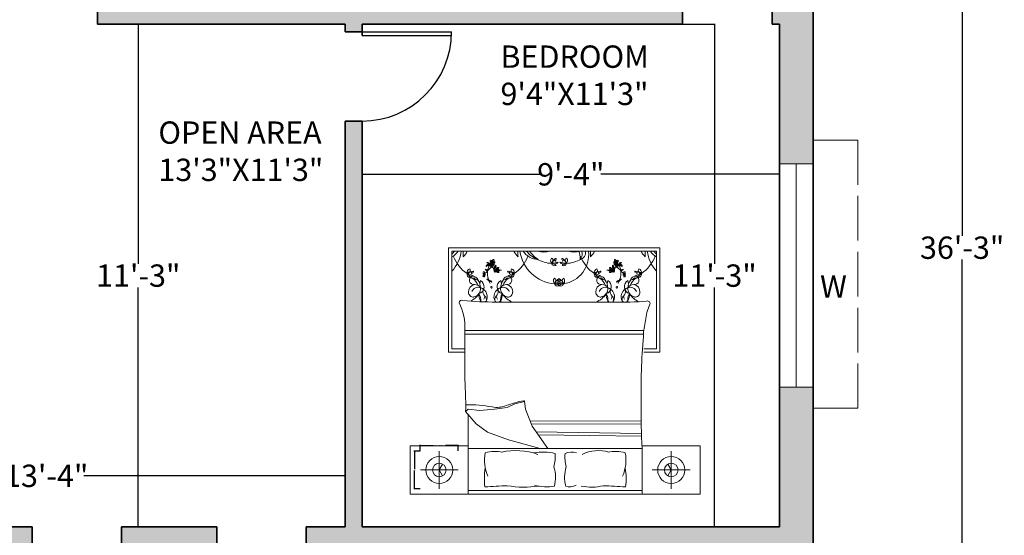
# Model space of a CAD drawing. Units: inches. Extents: x -5 to 482, y -460 to 66.
# Tile 16 of 31: x 218 to 482, y -282 to -143. Entities that reach past the tile are written whole.
import ezdxf

# ---------------------------------------------------------------- set-up
doc = ezdxf.new("R2010")
doc.units = ezdxf.units.IN
doc.header["$MEASUREMENT"] = 0
doc.linetypes.add('ACAD_ISO02W100', pattern=[15, 12, -3])
for name, color, linetype, lineweight in [('A-ANNO-DIMS', 2, 'Continuous', 18), ('A-ANNO-TEXT', 7, 'Continuous', 18), ('A-AREA-IDEN', 7, 'Continuous', 18), ('A-DOOR', 3, 'Continuous', 25), ('A-FURN', 8, 'Continuous', 18), ('A-GLAZ', 4, 'Continuous', 18), ('A-GLAZ-OVHD', 4, 'ACAD_ISO02W100', 13), ('A-WALL', 7, 'Continuous', 35), ('A-WALL-PATT', 152, 'Continuous', 13)]:
    doc.layers.add(name, color=color, linetype=linetype, lineweight=lineweight)
doc.styles.get("Standard").update_dxf_attribs({"font": 'arial.ttf'})
doc.dimstyles.get("Standard").update_dxf_attribs({"dimtxt": 0.18, "dimasz": 0.18, "dimexe": 0.18, "dimexo": 0.0625, "dimgap": 0.09, "dimtad": 0, "dimtih": 1, "dimtoh": 1, "dimdec": 0, "dimzin": 0, "dimdsep": 46, "dimlunit": 3, "dimtxsty": 'Standard', "dimcen": 0.09, "dimadec": 0, "dimazin": 0, "dimtfac": 1, "dimtdec": 0, "dimtofl": 0, "dimtmove": 0, "dimatfit": 3, "dimfxl": 1, "dimtolj": 1, "dimtzin": 0, "dimarcsym": 0})

# ---------------------------------------------------------------- blocks, each defined once
blk = doc.blocks.new('*D4')
at = {"layer": 'A-ANNO-DIMS', "color": 0, "lineweight": -2, "transparency": 16777216}
for p, q in [((430.44, 13.15), (470.55, 13.15)), ((470.37, 12.97), (470.37, -201.19)), ((470.37, -421.67), (470.37, -207.5)), ((430.44, -421.85), (470.55, -421.85))]:
    blk.add_line(p, q, dxfattribs=at)
at = {"layer": 'A-ANNO-DIMS', "color": 0, "transparency": 16777216}
for points in [[(470.34, 12.97), (470.4, 12.97), (470.37, 13.15)], [(470.34, -421.67), (470.4, -421.67), (470.37, -421.85)]]:
    blk.add_solid(points, dxfattribs=at)
at = {"layer": 'Defpoints', "color": 0, "transparency": 16777216}
for p in [(430.38, 13.15), (430.38, -421.85), (470.37, -421.85)]:
    blk.add_point(p, dxfattribs=at)
at = {"layer": 'A-ANNO-DIMS', "color": 0, "transparency": 16777216, "insert": (470.37, -204.35), "char_height": 6, "attachment_point": 5}
blk.add_mtext('\\A1;36\'-3"', dxfattribs=at)
blk = doc.blocks.new('*D15')
at = {"layer": 'A-ANNO-DIMS', "color": 0, "lineweight": -2, "transparency": 16777216}
for p, q in [((309.38, -184.91), (309.38, -184.46)), ((309.56, -184.64), (357.31, -184.64)), ((421.2, -184.64), (373.44, -184.64)), ((421.38, -184.91), (421.38, -184.46))]:
    blk.add_line(p, q, dxfattribs=at)
at = {"layer": 'A-ANNO-DIMS', "color": 0, "transparency": 16777216}
for points in [[(309.56, -184.61), (309.56, -184.67), (309.38, -184.64)], [(421.2, -184.61), (421.2, -184.67), (421.38, -184.64)]]:
    blk.add_solid(points, dxfattribs=at)
at = {"layer": 'Defpoints', "color": 0, "transparency": 16777216}
for p in [(421.38, -184.64), (309.38, -184.98), (421.38, -184.98)]:
    blk.add_point(p, dxfattribs=at)
at = {"layer": 'A-ANNO-DIMS', "color": 0, "transparency": 16777216, "insert": (365.38, -184.64), "char_height": 6, "attachment_point": 5}
blk.add_mtext('\\A1;9\'-4"', dxfattribs=at)
blk = doc.blocks.new('*D16')
at = {"layer": 'A-ANNO-DIMS', "color": 0, "lineweight": -2, "transparency": 16777216}
for p, q in [((395.44, -144.35), (404.13, -144.35)), ((403.95, -144.53), (403.95, -208.69)), ((403.95, -279.17), (403.95, -215)), ((395.44, -279.35), (404.13, -279.35))]:
    blk.add_line(p, q, dxfattribs=at)
at = {"layer": 'A-ANNO-DIMS', "color": 0, "transparency": 16777216}
for points in [[(403.92, -144.53), (403.98, -144.53), (403.95, -144.35)], [(403.92, -279.17), (403.98, -279.17), (403.95, -279.35)]]:
    blk.add_solid(points, dxfattribs=at)
at = {"layer": 'Defpoints', "color": 0, "transparency": 16777216}
for p in [(395.38, -144.35), (395.38, -279.35), (403.95, -279.35)]:
    blk.add_point(p, dxfattribs=at)
at = {"layer": 'A-ANNO-DIMS', "color": 0, "transparency": 16777216, "insert": (403.95, -211.85), "char_height": 6, "attachment_point": 5}
blk.add_mtext('\\A1;11\'-3"', dxfattribs=at)
blk = doc.blocks.new('*D17')
at = {"layer": 'A-ANNO-DIMS', "color": 0, "lineweight": -2, "transparency": 16777216}
for p, q in [((238.44, -144.35), (249.52, -144.35)), ((249.34, -144.53), (249.34, -208.69)), ((249.34, -279.17), (249.34, -215)), ((244.94, -279.35), (249.52, -279.35))]:
    blk.add_line(p, q, dxfattribs=at)
at = {"layer": 'A-ANNO-DIMS', "color": 0, "transparency": 16777216}
for points in [[(249.31, -144.53), (249.37, -144.53), (249.34, -144.35)], [(249.31, -279.17), (249.37, -279.17), (249.34, -279.35)]]:
    blk.add_solid(points, dxfattribs=at)
at = {"layer": 'Defpoints', "color": 0, "transparency": 16777216}
for p in [(238.38, -144.35), (244.88, -279.35), (249.34, -279.35)]:
    blk.add_point(p, dxfattribs=at)
at = {"layer": 'A-ANNO-DIMS', "color": 0, "transparency": 16777216, "insert": (249.34, -211.85), "char_height": 6, "attachment_point": 5}
blk.add_mtext('\\A1;11\'-3"', dxfattribs=at)
blk = doc.blocks.new('*D20')
at = {"layer": 'A-ANNO-DIMS', "color": 0, "lineweight": -2, "transparency": 16777216}
for p, q in [((144.41, -279.11), (144.41, -265.44)), ((144.59, -265.62), (214.53, -265.62)), ((304.7, -265.62), (234.75, -265.62)), ((304.88, -279.11), (304.88, -265.44))]:
    blk.add_line(p, q, dxfattribs=at)
at = {"layer": 'A-ANNO-DIMS', "color": 0, "transparency": 16777216}
for points in [[(144.59, -265.59), (144.59, -265.65), (144.41, -265.62)], [(304.7, -265.59), (304.7, -265.65), (304.88, -265.62)]]:
    blk.add_solid(points, dxfattribs=at)
at = {"layer": 'Defpoints', "color": 0, "transparency": 16777216}
for p in [(304.88, -265.62), (144.41, -279.17), (304.88, -279.17)]:
    blk.add_point(p, dxfattribs=at)
at = {"layer": 'A-ANNO-DIMS', "color": 0, "transparency": 16777216, "insert": (224.64, -265.62), "char_height": 6, "attachment_point": 5}
blk.add_mtext('\\A1;13\'-4"', dxfattribs=at)
blk = doc.blocks.new('DOOR-SWING-24IN')
for p, q in [((24, 1), (0, 1)), ((24, 0), (0, 0))]:
    blk.add_line(p, q)
blk.add_arc((24, 0), 24, 90, 180)
blk = doc.blocks.new('WIN-GLAZ-60IN')
for p, q in [((0, 9), (60, 9)), ((0, 4.5), (60, 4.5)), ((60, 0), (0, 0))]:
    blk.add_line(p, q)
blk = doc.blocks.new('WIN-SHADE-72IN')
for p, q in [((0, 12), (72, 12)), ((0, 12), (0, 0)), ((72, 12), (72, 0))]:
    blk.add_line(p, q)
blk = doc.blocks.new('BEDSIDE-LAMP-7IN')
for p, q in [((5.08, 10.16), (5.08, 0)), ((0, 5.08), (10.16, 5.08))]:
    blk.add_line(p, q)
for points in [[(5.08, 5.08), (4.17, 6.65)], [(5.08, 5.08), (4.17, 3.51)]]:
    blk.add_lwpolyline(points)
for radius in [3.63, 1.82]:
    blk.add_circle((5.08, 5.08), radius)
blk = doc.blocks.new('*D59')
at = {"layer": 'A-ANNO-DIMS', "color": 0, "lineweight": -2, "transparency": 16777216}
for p, q in [((325, -258.91), (325, -257.27)), ((325.18, -257.45), (328.41, -257.45)), ((334.99, -257.45), (331.75, -257.45)), ((335.17, -258.91), (335.17, -257.27))]:
    blk.add_line(p, q, dxfattribs=at)
at = {"layer": 'A-ANNO-DIMS', "color": 0, "transparency": 16777216}
for points in [[(325.18, -257.42), (325.18, -257.48), (325, -257.45)], [(334.99, -257.42), (334.99, -257.48), (335.17, -257.45)]]:
    blk.add_solid(points, dxfattribs=at)
at = {"layer": 'Defpoints', "color": 0, "transparency": 16777216}
for p in [(325, -257.45), (325, -258.97), (335.17, -258.97)]:
    blk.add_point(p, dxfattribs=at)
at = {"layer": 'A-ANNO-DIMS', "color": 0, "transparency": 16777216, "insert": (330.08, -257.45), "char_height": 0.18, "attachment_point": 5}
blk.add_mtext('\\A1;BEDSIDE LAMP 0\'-10" TYP.', dxfattribs=at)
blk = doc.blocks.new('*D60')
at = {"layer": 'A-ANNO-DIMS', "color": 0, "lineweight": -2, "transparency": 16777216}
for p, q in [((324.94, -258.97), (323.3, -258.97)), ((323.48, -259.15), (323.48, -263.87)), ((323.48, -268.96), (323.48, -264.23)), ((324.94, -269.14), (323.3, -269.14))]:
    blk.add_line(p, q, dxfattribs=at)
at = {"layer": 'A-ANNO-DIMS', "color": 0, "transparency": 16777216}
for points in [[(323.45, -259.15), (323.51, -259.15), (323.48, -258.97)], [(323.45, -268.96), (323.51, -268.96), (323.48, -269.14)]]:
    blk.add_solid(points, dxfattribs=at)
at = {"layer": 'Defpoints', "color": 0, "transparency": 16777216}
for p in [(325, -258.97), (323.48, -269.14), (325, -269.14)]:
    blk.add_point(p, dxfattribs=at)
at = {"layer": 'A-ANNO-DIMS', "color": 0, "transparency": 16777216, "insert": (323.48, -264.05), "char_height": 0.18, "attachment_point": 5}
blk.add_mtext('\\A1;0\'-10" TYP.', dxfattribs=at)

msp = doc.modelspace()

# ---------------------------------------------------------------- hatches: boundary and pattern name
at = {"layer": 'A-WALL-PATT'}
h = msp.add_hatch(color=256, dxfattribs=at)
h.dxf.hatch_style = 1
h.paths.add_polyline_path([(149.38, -412.85), (144.38, -412.85), (144.38, -283.85), (144.38, -279.35), (133.88, -279.35), (133.88, -283.85), (139.88, -283.85), (139.88, -412.85), (133.51, -412.85), (133.51, -413.92), (102.65, -413.92), (102.65, -421.02), (133.51, -421.02), (133.51, -421.85), (149.38, -421.85)])
h.paths.add_polyline_path([(226.05, -412.85), (218.88, -412.85), (218.88, -350.85), (262.88, -350.85), (262.88, -386.85), (267.38, -386.85), (267.38, -283.85), (270.38, -283.85), (270.38, -279.35), (244.88, -279.35), (244.88, -283.85), (262.88, -283.85), (262.88, -346.35), (218.88, -346.35), (218.88, -283.85), (220.88, -283.85), (220.88, -279.35), (214.38, -279.35), (214.38, -283.85), (214.38, -412.85), (209.38, -412.85), (209.38, -421.85), (226.05, -421.85)])
h.paths.add_polyline_path([(315.81, -412.85), (250.05, -412.85), (250.05, -421.85), (315.81, -421.85)])
h.paths.add_polyline_path([(430.38, -378.35), (421.38, -378.35), (421.38, -412.85), (375.81, -412.85), (375.81, -421.85), (430.38, -421.85)])
h.paths.add_polyline_path([(78.69, -413.92), (47.68, -413.92), (47.68, -412.85), (41.88, -412.85), (41.88, -283.85), (109.88, -283.85), (109.88, -279.35), (41.88, -279.35), (41.88, -241.85), (32.88, -241.85), (32.88, -421.85), (47.68, -421.85), (47.68, -421.02), (78.69, -421.02)])
h.paths.add_polyline_path([(41.88, -144.35), (154.38, -144.35), (154.38, -137.85), (149.88, -137.85), (149.88, -139.85), (41.88, -139.85), (41.88, -97.85), (32.88, -97.85), (32.88, -181.85), (41.88, -181.85)])
h.paths.add_polyline_path([(430.38, -241.85), (421.38, -241.85), (421.38, -279.35), (309.38, -279.35), (309.38, -170.35), (304.88, -170.35), (304.88, -279.35), (294.38, -279.35), (294.38, -283.85), (421.38, -283.85), (421.38, -318.35), (430.38, -318.35)])
h.paths.add_polyline_path([(430.38, -119.85), (421.38, -119.85), (421.38, -139.85), (419.38, -139.85), (419.38, -144.35), (421.38, -144.35), (421.38, -181.85), (430.38, -181.85)])
h.paths.add_polyline_path([(395.38, -139.85), (377.38, -139.85), (377.38, -75.85), (421.38, -75.85), (421.38, -95.85), (430.38, -95.85), (430.38, -45.6), (421.38, -45.6), (421.38, -71.35), (377.38, -71.35), (377.38, -22.85), (372.88, -22.85), (372.88, -139.85), (242.88, -139.85), (242.88, -137.85), (238.38, -137.85), (238.38, -144.35), (304.88, -144.35), (304.88, -146.35), (309.38, -146.35), (309.38, -144.35), (395.38, -144.35)])
h.paths.add_polyline_path([(65.88, 13.15), (32.88, 13.15), (32.88, -37.85), (41.88, -37.85), (41.88, 4.15), (65.88, 4.15)])
h.paths.add_polyline_path([(166.38, 13.15), (125.88, 13.15), (125.88, 4.15), (149.88, 4.15), (149.88, -113.85), (154.38, -113.85), (154.38, 4.15), (166.38, 4.15)])
h.paths.add_polyline_path([(277.88, 13.15), (226.38, 13.15), (226.38, 4.15), (238.38, 4.15), (238.38, -113.85), (242.88, -113.85), (242.88, 4.15), (277.88, 4.15)])
h.paths.add_polyline_path([(430.38, 13.15), (337.88, 13.15), (337.88, 4.15), (372.88, 4.15), (372.88, 1.15), (377.38, 1.15), (377.38, 4.15), (421.38, 4.15), (421.38, -21.6), (430.38, -21.6)])

# ---------------------------------------------------------------- linework, layer by layer
at = {"layer": 'A-FURN'}
for p, q in [((332.57, -204.38), (332.57, -232.4)), ((389.29, -204.38), (332.57, -204.38)), ((333.47, -205.28), (388.39, -205.28)), ((333.47, -231.5), (333.47, -205.28)), ((388.39, -205.28), (388.39, -231.5)), ((389.29, -232.4), (389.29, -204.38)), ((341.14, -213.17), (340.97, -214.04)), ((346.58, -213.17), (346.75, -214.04)), ((375.28, -213.17), (375.11, -214.04)), ((380.72, -213.17), (380.89, -214.04)), ((376.99, -218.94), (345.41, -218.94)), ((384.97, -226.58), (336.97, -226.58)), ((384.89, -227.55), (336.97, -227.55)), ((332.57, -232.4), (336.97, -232.4)), ((336.97, -231.5), (333.47, -231.5)), ((388.39, -231.5), (384.96, -231.5)), ((384.97, -232.4), (389.29, -232.4)), ((337.8, -247.74), (337.17, -248.37)), ((340.95, -248.06), (337.8, -247.74)), ((344.89, -247.74), (340.95, -248.06)), ((348.35, -247.27), (344.89, -247.74)), ((350.4, -246.32), (348.35, -247.27)), ((352.92, -245.69), (350.4, -246.32)), ((353.24, -247.74), (352.92, -245.69)), ((354.97, -252.31), (353.24, -247.74)), ((337.17, -248.37), (340, -251.68)), ((337.86, -270.54), (337.86, -249.18)), ((384.26, -250.96), (354.41, -250.84)), ((340, -251.68), (343, -253.88)), ((384.26, -251.76), (354.72, -251.64)), ((359.23, -258.24), (354.97, -252.31)), ((343, -253.88), (348.67, -255.93)), ((348.67, -255.93), (357.15, -258.24)), ((384.3, -254.21), (356.05, -253.81)), ((384.33, -255.01), (356.63, -254.62)), ((337.86, -258.24), (384.54, -258.24)), ((322.3, -270.54), (400.1, -270.54)), ((384.54, -269.54), (337.86, -269.54))]:
    msp.add_line(p, q, dxfattribs=at)
for points in [[(337, -241.25, -0.001242), (336.97, -226.49, 0.127202), (335.41, -219.13)], [(384.87, -228.16, -0.056112), (385.44, -223.88, -0.095341), (386.53, -219.76)], [(342.33, -268.6, -0.074897), (342.43, -263.52, 0.472817)], [(360.84, -263.23, -0.14099), (360.99, -268.41, -0.235245)], [(364.16, -263.23, 0.14099), (364, -268.41, 0.235245)], [(380.07, -268.6, 0.074897), (379.98, -263.52, -0.472817)]]:
    msp.add_lwpolyline(points, format="xyb", dxfattribs=at)
for points in [[(337.86, -257.57), (322.3, -257.57), (322.3, -270.54)], [(384.54, -270.54), (384.54, -257.57), (400.1, -257.57), (400.1, -270.54)]]:
    msp.add_lwpolyline(points, dxfattribs=at)
for centre in [(344.34, -208.26), (377.52, -208.26), (345.63, -210.35), (376.22, -210.35)]:
    msp.add_circle(centre, 0.198, dxfattribs=at)
for centre, radius, start, end in [((329.23, -201.63), 6.17, 313.5186, 323.6964), ((331.01, -202.55), 4.95, 299.8884, 326.5383), ((325.91, -203.91), 10.16, 318.1144, 352.255), ((333.78, -203.69), 4.13, 311.0454, 337.4453), ((322.46, -205.91), 14.06, 356.3481, 2.5919), ((353.94, -203.69), 4.13, 202.5547, 228.9546), ((365.25, -205.91), 14.06, 177.4081, 183.6519), ((361.81, -203.91), 10.16, 187.745, 265.5377), ((356.71, -202.55), 4.95, 213.4617, 268.728), ((358.49, -201.63), 6.17, 216.3036, 252.1496), ((361.73, -199.89), 9.18, 215.947, 235.9877), ((358.19, -199.94), 5.59, 252.9798, 286.4569), ((360.4, -197.06), 8.26, 264.3643, 265.6213), ((364.75, -191.4), 14.76, 250.0972, 250.2783), ((362.32, -206.26), 7.86, 278.1803, 7.1364), ((366.27, -199.94), 5.59, 253.5431, 287.0202), ((364.05, -197.06), 8.26, 274.3787, 275.6357), ((359.7, -191.4), 14.76, 289.7217, 289.9028), ((363.33, -206.97), 4.55, 353.3805, 21.883), ((367.51, -205.71), 1.82, 280.9261, 13.6102), ((366.14, -205.96), 2.31, 318.0951, 17.1391), ((356.61, -205.91), 14.06, 356.3481, 2.5919), ((367.92, -203.69), 4.13, 311.0454, 337.4453), ((388.08, -203.69), 4.13, 202.5547, 228.9546), ((399.39, -205.91), 14.06, 177.4081, 183.6519), ((395.95, -203.91), 10.16, 187.745, 221.8856), ((390.85, -202.55), 4.95, 213.4617, 240.1116), ((392.63, -201.63), 6.17, 216.3036, 226.4814), ((343.29, -202.91), 10.16, 201.4092, 235.6135), ((343.06, -208.55), 0.221, 55.6077, 145.6462), ((342.91, -209.02), 0.599, 21.7087, 93.0299), ((339.75, -213.29), 5.79, 53.6254, 57.3216), ((343.09, -208.87), 0.516, 342.8042, 79.6943), ((343.05, -208.82), 0.229, 338.2452, 53.6254), ((346.26, -210.84), 3.23, 137.5083, 145.9967), ((343.92, -207.89), 0.196, 134.3732, 211.9501), ((344.29, -207.66), 0.625, 211.9501, 255.2442), ((343.93, -208.11), 0.391, 8.5614, 112.5914), ((344.12, -208.53), 0.27, 88.5719, 233.8954), ((344.09, -208.61), 0.194, 228.2946, 6.2474), ((344.04, -208.09), 0.131, 352.868, 97.094), ((343.91, -208.38), 0.273, 298.8493, 359.9355), ((343.97, -208.61), 0.312, 4.2123, 48.1587), ((344.61, -207.89), 0.327, 100.9597, 208.7804), ((344.61, -208.57), 0.33, 183.635, 258.4363), ((344.57, -208.45), 0.189, 178.1325, 268.8919), ((344.96, -208.33), 0.602, 132.3896, 156.5724), ((344.7, -208.4), 0.324, 42.3208, 130.2111), ((344.77, -208.07), 0.41, 226.3462, 279.6513), ((344.33, -207.72), 0.46, 291.6382, 4.947), ((344.35, -208.82), 0.476, 7.4968, 71.2737), ((344.69, -207.64), 0.649, 254.2829, 276.9148), ((344.64, -207.69), 0.152, 4.947, 127.5263), ((344.81, -208.3), 0.171, 279.6513, 42.3208), ((344.43, -202.91), 10.16, 304.3865, 338.5908), ((361.03, -198.47), 10.16, 242.5854, 265.5377), ((361.07, -207.84), 1.13, 140.8855, 222.2127), ((359.79, -207.87), 0.848, 301.6373, 61.4609), ((362.67, -209.43), 2.57, 121.989, 161.0841), ((361.07, -208.56), 0.831, 76.148, 182.2415), ((362.36, -215.38), 7.11, 92.7418, 107.407), ((360.9, -207.13), 1.61, 245.6899, 314.4589), ((360.19, -210.33), 1.74, 44.6273, 88.5415), ((361.05, -208.36), 0.842, 196.1963, 296.9726), ((361.24, -207.86), 0.11, 140.0755, 76.148), ((361.37, -207.36), 0.126, 288.4408, 121.989), ((361.39, -207.42), 0.0613, 171.9833, 288.4408), ((362.09, -215.38), 7.11, 72.593, 87.2582), ((363.55, -207.13), 1.61, 225.5411, 294.3101), ((363.08, -207.36), 0.126, 58.011, 251.5592), ((364.26, -210.33), 1.74, 91.4585, 135.3727), ((363.41, -208.36), 0.842, 243.0274, 343.8037), ((363.06, -207.42), 0.0613, 251.5592, 8.0167), ((363.2, -207.91), 0.0662, 103.9791, 39.8091), ((361.78, -209.43), 2.57, 18.9159, 58.011), ((363.38, -208.56), 0.831, 357.7585, 103.852), ((364.66, -207.87), 0.848, 118.5391, 238.3627), ((363.38, -207.84), 1.13, 317.7873, 39.1145), ((363.42, -198.47), 10.16, 274.4623, 297.4146), ((377.43, -202.91), 10.16, 201.4092, 235.6135), ((377.05, -208.3), 0.171, 137.6792, 260.3487), ((377.16, -208.4), 0.324, 49.7889, 137.6792), ((377.09, -208.07), 0.41, 260.3487, 313.6538), ((377.51, -208.82), 0.476, 108.7263, 172.5032), ((377.22, -207.69), 0.152, 52.4737, 175.053), ((377.53, -207.72), 0.46, 175.053, 248.3618), ((377.17, -207.64), 0.649, 263.0852, 285.7171), ((377.29, -208.45), 0.189, 271.1081, 1.8675), ((376.9, -208.33), 0.602, 23.4276, 47.6104), ((377.25, -207.89), 0.327, 331.2196, 79.0403), ((377.25, -208.57), 0.33, 281.5637, 356.365), ((377.92, -208.11), 0.391, 67.4086, 171.4386), ((377.89, -208.61), 0.312, 131.8413, 175.7877), ((377.77, -208.61), 0.194, 173.7526, 311.7054), ((377.81, -208.09), 0.131, 82.906, 187.132), ((377.95, -208.38), 0.273, 180.0645, 241.1507), ((377.57, -207.66), 0.625, 284.7558, 328.0499), ((377.74, -208.53), 0.27, 306.1046, 91.4281), ((375.59, -210.84), 3.23, 34.0033, 42.4917), ((377.94, -207.89), 0.196, 328.0499, 45.6268), ((378.77, -208.87), 0.516, 100.3057, 197.1958), ((378.95, -209.02), 0.599, 86.9701, 158.2913), ((378.81, -208.82), 0.229, 126.3746, 201.7548), ((378.8, -208.55), 0.221, 34.3538, 124.3923), ((382.11, -213.29), 5.79, 122.6784, 126.3746), ((378.57, -202.91), 10.16, 304.3865, 338.5908), ((338.65, -211.05), 1.13, 110.9613, 192.2885), ((338.37, -211.49), 0.842, 166.272, 267.0484), ((337.53, -210.44), 0.848, 271.7131, 31.5367), ((339.24, -213.22), 2.57, 92.0648, 131.1598), ((338.29, -211.67), 0.831, 46.2238, 152.3173), ((336.01, -218.23), 7.11, 62.8176, 77.4827), ((338.86, -210.35), 1.61, 215.7657, 284.5347), ((336.65, -212.77), 1.74, 14.7031, 58.6173), ((338.79, -211.15), 0.11, 110.2817, 46.2238), ((339.14, -210.85), 0.0613, 142.0591, 258.5166), ((339.16, -210.78), 0.126, 258.5166, 92.0648), ((342.06, -211.16), 0.327, 100.9597, 142.2379), ((342.42, -211.59), 0.602, 132.3896, 156.5724), ((341.79, -210.98), 0.46, 291.6382, 4.947), ((342.09, -210.96), 0.152, 4.947, 127.5263), ((337.66, -205.53), 7.39, 307.9541, 316.8459), ((342.45, -212.36), 2.19, 82.8698, 91.6736), ((342.76, -209.99), 0.408, 205.5379, 258.6744), ((342.17, -211.37), 1.23, 59.344, 79.7412), ((342.9, -209.27), 0.221, 123.0979, 213.1364), ((341.91, -211.37), 1.25, 43.6929, 51.7899), ((343.28, -209.59), 0.599, 92.3172, 160.5201), ((346.02, -214.14), 5.79, 121.1156, 124.8118), ((342.67, -210.55), 0.373, 355.7131, 81.6568), ((343.21, -209.37), 0.516, 82.6008, 147.1845), ((342.47, -210.88), 0.652, 27.3659, 59.344), ((342.96, -210.45), 0.159, 202.5583, 304.2343), ((343.14, -209.38), 0.229, 45.7354, 121.1156), ((349.47, -211.01), 6.44, 176.1723, 196.4158), ((346.26, -210.84), 3.23, 150.7959, 175.244), ((350.91, -217.72), 10.63, 127.8256, 137.7588), ((343.42, -208.97), 0.173, 158.2452, 340.6395), ((343.42, -209.1), 0.173, 225.7354, 48.1297), ((346.67, -207.52), 3.45, 201.7087, 206.2181), ((343.93, -209.88), 0.903, 40.9365, 112.7695), ((343.63, -209.58), 0.531, 49.3812, 95.5456), ((344.02, -209.37), 0.549, 61.1838, 141.6792), ((346.6, -206.55), 3.87, 220.182, 239.456), ((344.39, -208.69), 0.639, 229.3812, 289.9959), ((343.98, -209.47), 0.656, 15.6484, 62.2957), ((344.67, -208.8), 0.153, 215.0752, 14.7644), ((344.35, -209.04), 0.903, 287.889, 359.722), ((344.32, -209.46), 0.531, 305.1128, 351.2773), ((344.6, -210.44), 0.549, 3.8774, 87.1501), ((344.21, -210.23), 0.531, 352.0748, 38.2393), ((344.12, -210.64), 0.903, 343.6301, 55.4631), ((345.37, -210.39), 0.639, 172.0748, 232.6895), ((344.76, -209.37), 0.549, 271.4625, 339.4747), ((345.48, -209.64), 0.639, 110.6625, 171.2773), ((344.49, -210.46), 0.656, 318.342, 4.9894), ((345.22, -209.98), 0.196, 134.3732, 211.9501), ((346.6, -206.55), 3.87, 246.1523, 246.9499), ((345.58, -209.75), 0.625, 211.9501, 255.2442), ((345.23, -210.2), 0.391, 8.5614, 112.5914), ((345.42, -210.62), 0.27, 88.5719, 233.8954), ((344.66, -209.32), 0.656, 338.3627, 25.0101), ((345.39, -210.7), 0.194, 228.2946, 6.2474), ((345.34, -210.18), 0.131, 352.868, 97.094), ((345.2, -210.47), 0.273, 298.8493, 359.9355), ((345.27, -210.7), 0.312, 4.2123, 48.1587), ((345.9, -209.98), 0.327, 100.9597, 208.7804), ((345.91, -210.65), 0.33, 183.635, 258.4363), ((345.86, -210.53), 0.189, 178.1325, 268.8919), ((346.26, -210.42), 0.602, 132.3896, 156.5724), ((345.99, -210.49), 0.324, 42.3208, 130.2111), ((346.07, -210.15), 0.41, 226.3462, 279.6513), ((345.63, -209.81), 0.46, 291.6382, 4.947), ((345.64, -210.91), 0.476, 7.4968, 71.2737), ((345.99, -209.73), 0.649, 254.2829, 276.9148), ((345.93, -209.78), 0.152, 4.947, 127.5263), ((345.97, -210.89), 0.153, 215.0752, 14.7644), ((346.11, -210.39), 0.171, 279.6513, 42.3208), ((346.6, -206.55), 3.87, 265.2415, 272.8929), ((348.56, -210.78), 0.126, 87.9352, 281.4834), ((348.86, -210.35), 1.61, 255.4653, 324.2343), ((351.7, -218.23), 7.11, 102.5173, 117.1824), ((348.47, -213.22), 2.57, 48.8402, 87.9352), ((348.57, -210.85), 0.0613, 281.4834, 37.9409), ((349.43, -211.67), 0.831, 27.6827, 133.7762), ((348.94, -211.2), 0.0662, 133.7729, 69.7333), ((350.19, -210.44), 0.848, 148.4633, 268.2869), ((349.34, -211.49), 0.842, 272.9516, 13.728), ((351.07, -212.77), 1.74, 121.3827, 165.2969), ((349.06, -211.05), 1.13, 347.7115, 69.0387), ((372.8, -211.05), 1.13, 110.9613, 192.2885), ((372.51, -211.49), 0.842, 166.272, 267.0484), ((371.67, -210.44), 0.848, 271.7131, 31.5367), ((373.39, -213.22), 2.57, 92.0648, 131.1598), ((372.43, -211.67), 0.831, 46.2238, 152.3173), ((370.79, -212.77), 1.74, 14.7031, 58.6173), ((373, -210.35), 1.61, 215.7657, 284.5347), ((370.16, -218.23), 7.11, 62.8176, 77.4827), ((372.93, -211.15), 0.11, 110.2817, 46.2238), ((373.29, -210.85), 0.0613, 142.0591, 258.5166), ((373.3, -210.78), 0.126, 258.5166, 92.0648), ((375.26, -206.55), 3.87, 267.1071, 274.7585), ((375.75, -210.39), 0.171, 137.6792, 260.3487), ((375.87, -210.49), 0.324, 49.7889, 137.6792), ((375.79, -210.15), 0.41, 260.3487, 313.6538), ((376.22, -210.91), 0.476, 108.7263, 172.5032), ((375.89, -210.89), 0.153, 165.2356, 324.9248), ((375.92, -209.78), 0.152, 52.4737, 175.053), ((376.23, -209.81), 0.46, 175.053, 248.3618), ((375.87, -209.73), 0.649, 263.0852, 285.7171), ((375.99, -210.53), 0.189, 271.1081, 1.8675), ((375.6, -210.42), 0.602, 23.4276, 47.6104), ((375.95, -209.98), 0.327, 331.2196, 79.0403), ((375.95, -210.65), 0.33, 281.5637, 356.365), ((376.63, -210.2), 0.391, 67.4086, 171.4386), ((376.59, -210.7), 0.312, 131.8413, 175.7877), ((376.47, -210.7), 0.194, 173.7526, 311.7054), ((376.66, -210.47), 0.273, 180.0645, 241.1507), ((376.52, -210.18), 0.131, 82.906, 187.132), ((376.28, -209.75), 0.625, 284.7558, 328.0499), ((376.44, -210.62), 0.27, 306.1046, 91.4281), ((377.2, -209.32), 0.656, 154.9899, 201.6373), ((377.1, -209.37), 0.549, 200.5253, 268.5375), ((377.51, -209.04), 0.903, 180.278, 252.111), ((376.38, -209.64), 0.639, 8.7227, 69.3375), ((377.26, -210.44), 0.549, 92.8499, 176.1226), ((377.37, -210.46), 0.656, 175.0106, 221.658), ((376.64, -209.98), 0.196, 328.0499, 45.6268), ((375.26, -206.55), 3.87, 293.0501, 293.8477), ((377.74, -210.64), 0.903, 124.5369, 196.3699), ((376.49, -210.39), 0.639, 307.3105, 7.9252), ((377.54, -209.46), 0.531, 188.7227, 234.8872), ((377.19, -208.8), 0.153, 165.2356, 324.9248), ((377.65, -210.23), 0.531, 141.7607, 187.9252), ((375.26, -206.55), 3.87, 300.544, 319.818), ((377.88, -209.47), 0.656, 117.7043, 164.3516), ((377.93, -209.88), 0.903, 67.2305, 139.0635), ((377.47, -208.69), 0.639, 250.0041, 310.6188), ((370.94, -217.72), 10.63, 42.2412, 52.1744), ((377.84, -209.37), 0.549, 38.3208, 118.8162), ((378.23, -209.58), 0.531, 84.4544, 130.6188), ((378.44, -209.1), 0.173, 131.8703, 314.2646), ((378.44, -208.97), 0.173, 199.3605, 21.7548), ((375.19, -207.52), 3.45, 333.7819, 338.2913), ((375.59, -210.84), 3.23, 4.756, 29.2041), ((378.72, -209.38), 0.229, 58.8844, 134.2646), ((372.39, -211.01), 6.44, 343.5842, 3.8277), ((378.65, -209.37), 0.516, 32.8155, 97.3992), ((378.58, -209.59), 0.599, 19.4799, 87.6828), ((379.19, -210.55), 0.373, 98.3432, 184.2869), ((379.39, -210.88), 0.652, 120.656, 152.6341), ((378.9, -210.45), 0.159, 235.7657, 337.4417), ((384.2, -205.53), 7.39, 223.1541, 232.0459), ((375.84, -214.14), 5.79, 55.1882, 58.8844), ((379.95, -211.37), 1.25, 128.2101, 136.3071), ((379.69, -211.37), 1.23, 100.2588, 120.656), ((378.96, -209.27), 0.221, 326.8636, 56.9021), ((379.4, -212.36), 2.19, 88.3264, 97.1302), ((379.1, -209.99), 0.408, 281.3256, 334.4621), ((379.77, -210.96), 0.152, 52.4737, 175.053), ((380.07, -210.98), 0.46, 175.053, 248.3618), ((379.44, -211.59), 0.602, 23.4276, 47.6104), ((379.8, -211.16), 0.327, 37.7621, 79.0403), ((382.7, -210.78), 0.126, 87.9352, 281.4834), ((385.85, -218.23), 7.11, 102.5173, 117.1824), ((383, -210.35), 1.61, 255.4653, 324.2343), ((382.61, -213.22), 2.57, 48.8402, 87.9352), ((382.72, -210.85), 0.0613, 281.4834, 37.9409), ((383.57, -211.67), 0.831, 27.6827, 133.7762), ((383.08, -211.2), 0.0662, 133.7729, 69.7333), ((384.33, -210.44), 0.848, 148.4633, 268.2869), ((385.21, -212.77), 1.74, 121.3827, 165.2969), ((383.49, -211.49), 0.842, 272.9516, 13.728), ((383.2, -211.05), 1.13, 347.7115, 69.0387), ((339.36, -213.1), 1.17, 109.1312, 279.736), ((339.12, -211.84), 0.716, 216.7319, 296.0245), ((337.05, -215.67), 3.67, 18.2955, 58.7386), ((339.08, -213.45), 1.46, 15.6955, 94.031), ((340.65, -211.52), 1.55, 218.4175, 263.8338), ((337.01, -215.38), 4.17, 3.4924, 33.7117), ((340.18, -214.84), 1.93, 286.8663, 60.0915), ((341.79, -211.52), 0.198, 273.2768, 86.7232), ((342.07, -211.83), 0.33, 217.3642, 258.4363), ((342.02, -211.71), 0.189, 178.1325, 268.8919), ((342.15, -211.67), 0.324, 42.3208, 130.2111), ((342.23, -211.33), 0.41, 226.3462, 279.6513), ((341.8, -212.09), 0.476, 7.4968, 71.2737), ((342.15, -210.91), 0.649, 254.2829, 276.9148), ((342.13, -212.07), 0.153, 215.0752, 14.7644), ((342.27, -211.57), 0.171, 279.6513, 42.3208), ((342.92, -214.97), 2.19, 82.8698, 91.6736), ((343.22, -212.61), 0.408, 205.5379, 258.6744), ((342.63, -213.99), 1.23, 59.344, 79.7412), ((342.37, -213.99), 1.25, 43.6929, 51.7899), ((343.14, -213.17), 0.373, 355.7131, 81.6568), ((342.93, -213.49), 0.652, 27.3659, 59.344), ((343.42, -213.06), 0.159, 202.5583, 304.2343), ((349.47, -211.01), 6.44, 200.1059, 206.9968), ((343.71, -213.51), 0.373, 36.5232, 122.4668), ((343.52, -213.85), 0.652, 58.836, 90.8141), ((343.67, -213.21), 0.159, 173.9457, 275.6216), ((343.35, -214.57), 1.25, 66.3901, 74.4871), ((343.22, -214.34), 1.23, 38.4388, 58.836), ((344.16, -213.17), 0.408, 219.5056, 272.6421), ((342.22, -214.56), 2.19, 26.5064, 35.3102), ((347.54, -214.84), 1.93, 119.9085, 253.1337), ((350.71, -215.38), 4.17, 146.2883, 176.5076), ((350.67, -215.67), 3.67, 121.2614, 161.7045), ((348.64, -213.45), 1.46, 85.969, 164.3045), ((347.07, -211.52), 1.55, 276.1662, 321.5825), ((348.36, -213.1), 1.17, 260.264, 70.8688), ((348.6, -211.84), 0.716, 243.9755, 323.2681), ((361.85, -213.28), 1.13, 140.8855, 222.2127), ((360.57, -213.32), 0.848, 301.6373, 61.4609), ((361.85, -214.01), 0.831, 76.148, 182.2415), ((363.45, -214.87), 2.57, 121.989, 161.0841), ((361.68, -212.57), 1.61, 245.6899, 314.4589), ((363.14, -220.82), 7.11, 92.7418, 107.407), ((362.78, -212.57), 1.61, 225.5411, 294.3101), ((361.31, -220.82), 7.11, 72.593, 87.2582), ((362.02, -213.31), 0.11, 140.0755, 76.148), ((362.15, -212.8), 0.126, 288.4408, 121.989), ((362.17, -212.86), 0.0613, 171.9833, 288.4408), ((362.3, -212.8), 0.126, 58.011, 251.5592), ((362.28, -212.86), 0.0613, 251.5592, 8.0167), ((362.42, -213.35), 0.0662, 103.9791, 39.8091), ((361.01, -214.87), 2.57, 18.9159, 58.011), ((362.61, -214.01), 0.831, 357.7585, 103.852), ((363.88, -213.32), 0.848, 118.5391, 238.3627), ((362.6, -213.28), 1.13, 317.7873, 39.1145), ((373.5, -213.1), 1.17, 109.1312, 279.736), ((373.26, -211.84), 0.716, 216.7319, 296.0245), ((371.19, -215.67), 3.67, 18.2955, 58.7386), ((373.22, -213.45), 1.46, 15.6955, 94.031), ((374.79, -211.52), 1.55, 218.4175, 263.8338), ((371.15, -215.38), 4.17, 3.4924, 33.7117), ((374.32, -214.84), 1.93, 286.8663, 60.0915), ((378.64, -214.34), 1.23, 121.164, 141.5612), ((379.64, -214.56), 2.19, 144.6898, 153.4936), ((377.7, -213.17), 0.408, 267.3579, 320.4944), ((378.15, -213.51), 0.373, 57.5332, 143.4768), ((378.34, -213.85), 0.652, 89.1859, 121.164), ((378.51, -214.57), 1.25, 105.5129, 113.6099), ((372.39, -211.01), 6.44, 333.0032, 339.8941), ((378.19, -213.21), 0.159, 264.3784, 6.0543), ((378.72, -213.17), 0.373, 98.3432, 184.2869), ((378.93, -213.49), 0.652, 120.656, 152.6341), ((378.44, -213.06), 0.159, 235.7657, 337.4417), ((379.49, -213.99), 1.25, 128.2101, 136.3071), ((379.22, -213.99), 1.23, 100.2588, 120.656), ((378.94, -214.97), 2.19, 88.3264, 97.1302), ((378.64, -212.61), 0.408, 281.3256, 334.4621), ((379.59, -211.57), 0.171, 137.6792, 260.3487), ((379.71, -211.67), 0.324, 49.7889, 137.6792), ((379.63, -211.33), 0.41, 260.3487, 313.6538), ((380.06, -212.09), 0.476, 108.7263, 172.5032), ((379.73, -212.07), 0.153, 165.2356, 324.9248), ((379.71, -210.91), 0.649, 263.0852, 285.7171), ((381.68, -214.84), 1.93, 119.9085, 253.1337), ((379.83, -211.71), 0.189, 271.1081, 1.8675), ((379.79, -211.83), 0.33, 281.5637, 322.6358), ((380.07, -211.52), 0.198, 93.2768, 266.7232), ((384.85, -215.38), 4.17, 146.2883, 176.5076), ((384.81, -215.67), 3.67, 121.2614, 161.7045), ((382.78, -213.45), 1.46, 85.969, 164.3045), ((381.21, -211.52), 1.55, 276.1662, 321.5825), ((382.5, -213.1), 1.17, 260.264, 70.8688), ((382.74, -211.84), 0.716, 243.9755, 323.2681), ((339.79, -216.1), 1.86, 97.1143, 185.0551), ((339.25, -216.29), 1.31, 178.9462, 275.5144), ((340.52, -216.8), 1.81, 68.5779, 158.4181), ((338.85, -215.31), 2.34, 283.079, 4.7067), ((339.46, -216.51), 2.26, 35.9599, 87.6409), ((343.71, -216.96), 3, 143.6555, 147.2989), ((341.4, -215.66), 0.483, 344.8529, 102.6959), ((340.48, -217.52), 2.48, 330.8249, 70.7178), ((343.41, -216.2), 1.59, 164.8529, 228.4347), ((344.08, -214.92), 0.15, 79.5616, 257.2949), ((344.06, -215.02), 0.244, 259.5864, 79.5616), ((347.24, -217.52), 2.48, 109.2822, 209.1751), ((344.31, -216.2), 1.59, 311.5653, 15.1471), ((346.32, -215.66), 0.483, 77.3041, 195.1471), ((348.25, -216.51), 2.26, 92.3591, 144.0401), ((344.01, -216.96), 3, 32.7011, 36.3445), ((348.87, -215.31), 2.34, 175.2933, 256.921), ((347.2, -216.8), 1.81, 21.5819, 111.4221), ((347.93, -216.1), 1.86, 354.9449, 82.8857), ((348.47, -216.29), 1.31, 264.4856, 1.0538), ((361.82, -213.8), 0.842, 196.1963, 296.9726), ((360.97, -215.77), 1.74, 44.6273, 88.5415), ((362.63, -213.8), 0.842, 243.0274, 343.8037), ((363.48, -215.77), 1.74, 91.4585, 135.3727), ((373.93, -216.1), 1.86, 97.1143, 185.0551), ((373.39, -216.29), 1.31, 178.9462, 275.5144), ((374.66, -216.8), 1.81, 68.5779, 158.4181), ((372.99, -215.31), 2.34, 283.079, 4.7067), ((373.61, -216.51), 2.26, 35.9599, 87.6409), ((377.85, -216.96), 3, 143.6555, 147.2989), ((375.54, -215.66), 0.483, 344.8529, 102.6959), ((374.62, -217.52), 2.48, 330.8249, 70.7178), ((377.55, -216.2), 1.59, 164.8529, 228.4347), ((377.79, -215.02), 0.244, 100.4384, 280.4136), ((377.78, -214.92), 0.15, 282.7051, 100.4384), ((381.38, -217.52), 2.48, 109.2822, 209.1751), ((378.45, -216.2), 1.59, 311.5653, 15.1471), ((380.46, -215.66), 0.483, 77.3041, 195.1471), ((382.39, -216.51), 2.26, 92.3591, 144.0401), ((378.15, -216.96), 3, 32.7011, 36.3445), ((383.01, -215.31), 2.34, 175.2933, 256.921), ((381.34, -216.8), 1.81, 21.5819, 111.4221), ((382.07, -216.1), 1.86, 354.9449, 82.8857), ((382.61, -216.29), 1.31, 264.4856, 1.0538), ((336.12, -219.18), 0.718, 62.6588, 176.02), ((344.48, -137.96), 80.98, 264.3113, 270.6567), ((335.82, -213.46), 5.89, 296.7003, 326.3329), ((343.71, -216.96), 3, 175.2696, 214.215), ((337.98, -218.36), 3.22, 350.8446, 31.1782), ((341.97, -218.08), 0.937, 217.675, 239.9707), ((340.1, -217.08), 2.24, 330.0851, 352.564), ((341.57, -218.26), 1.16, 336.1646, 48.4347), ((341.97, -218.08), 0.937, 296.442, 315.5483), ((346.14, -218.26), 1.16, 131.5653, 203.8354), ((345.75, -218.08), 0.937, 224.4517, 246.771), ((347.62, -217.08), 2.24, 187.436, 209.9149), ((345.75, -218.08), 0.937, 293.2856, 322.325), ((344.01, -216.96), 3, 325.785, 4.7304), ((349.74, -218.36), 3.22, 148.8218, 190.2867), ((351.9, -213.46), 5.89, 213.6671, 248.5059), ((369.96, -213.46), 5.89, 291.4941, 326.3329), ((377.85, -216.96), 3, 175.2696, 214.215), ((372.12, -218.36), 3.22, 349.7133, 31.1782), ((376.11, -218.08), 0.937, 217.675, 246.7144), ((374.24, -217.08), 2.24, 330.0851, 352.564), ((376.11, -218.08), 0.937, 293.2856, 315.5483), ((375.72, -218.26), 1.16, 336.1646, 48.4347), ((379.38, -143.28), 75.7, 268.1965, 274.7598), ((380.28, -218.26), 1.16, 131.5653, 203.8354), ((379.89, -218.08), 0.937, 224.4517, 253.3657), ((381.76, -217.08), 2.24, 187.436, 209.9149), ((379.89, -218.08), 0.937, 287.4186, 322.325), ((378.15, -216.96), 3, 325.785, 4.7304), ((383.88, -218.36), 3.22, 148.8218, 190.751), ((386.04, -213.46), 5.89, 213.6671, 246.3547), ((385.94, -219.36), 0.709, 326.1736, 113.4781), ((566.55, -243.65), 182.34, 175.1265, 180.8855), ((265.84, -246.44), 71.35, 358.447, 4.1706), ((358.32, -275.09), 30.17, 100.6617, 109.8806), ((352.75, -245.63), 0.188, 340.2464, 91.1377), ((338.5, -275.92), 29.36, 78.6608, 92.5481), ((345.52, -240.92), 6.33, 258.6608, 293.7384), ((524, -248.73), 139.78, 179.0718, 183.9), ((350.59, -276.92), 18.08, 70.7385, 101.9603), ((372.8, -268.74), 9.9, 73.8254, 116.1239), ((352.24, -261.48), 10.03, 168.2417, 204.8684), ((345.11, -269.51), 10.43, 78.9631, 104.8961), ((357.91, -272.97), 13.72, 76.3762, 100.1383), ((351.67, -260.63), 9.53, 344.1707, 5.9871), ((373.33, -260.63), 9.53, 174.0129, 195.8293), ((365.59, -263.38), 4.12, 71.4593, 114.9817), ((377.3, -269.51), 10.43, 75.1039, 101.0369), ((370.16, -261.48), 10.03, 335.1316, 11.7583), ((385.21, -1008.93), 741.58, 92.85022, 93.31479), ((352.99, -240.45), 28.21, 260.503, 277.7804), ((358.95, -254.7), 13.86, 256.04, 278.4751), ((365.07, -264.72), 3.85, 253.8974, 296.6563), ((370.84, -254.98), 13.68, 258.8159, 283.6573), ((337.19, -1008.93), 741.58, 86.68521, 87.14978)]:
    msp.add_arc(centre, radius, start, end, dxfattribs=at)
at = {"layer": 'A-GLAZ'}
for p, q in [((430.38, -181.85), (421.38, -181.85)), ((421.38, -241.85), (430.38, -241.85))]:
    msp.add_line(p, q, dxfattribs=at)
at = {"layer": 'A-WALL'}
for p, q in [((430.38, 13.15), (430.38, -421.85)), ((238.38, -137.85), (238.38, -144.35)), ((395.38, -144.35), (395.38, -139.85)), ((419.38, -139.85), (419.38, -144.35)), ((238.38, -144.35), (304.88, -144.35)), ((304.88, -144.35), (304.88, -146.35)), ((309.38, -144.35), (309.38, -147.35)), ((309.38, -144.35), (395.38, -144.35)), ((419.38, -144.35), (421.38, -144.35)), ((421.38, -144.35), (421.38, -279.35)), ((309.38, -146.35), (304.88, -146.35)), ((304.88, -170.35), (309.38, -170.35)), ((304.88, -170.35), (304.88, -279.35)), ((309.38, -170.35), (309.38, -279.35)), ((214.38, -279.35), (220.88, -279.35)), ((220.88, -283.85), (220.88, -279.35)), ((244.88, -283.85), (244.88, -279.35)), ((244.88, -279.35), (270.38, -279.35)), ((270.38, -283.85), (270.38, -279.35)), ((294.38, -279.35), (294.38, -283.85)), ((294.38, -279.35), (304.88, -279.35)), ((309.38, -279.35), (421.38, -279.35))]:
    msp.add_line(p, q, dxfattribs=at)

# ---------------------------------------------------------------- block references
at = {"layer": 'A-DOOR', "rotation": 180}
msp.add_blockref('DOOR-SWING-24IN', (333.38, -146.35), dxfattribs=at)
at = {"layer": 'A-FURN', "rotation": 180}
msp.add_blockref('BEDSIDE-LAMP-7IN', (335.17, -258.97), dxfattribs=at)
at = {"layer": 'A-FURN'}
msp.add_blockref('BEDSIDE-LAMP-7IN', (387.24, -269.13), dxfattribs=at)
at = {"layer": 'A-GLAZ', "rotation": 90.00000000000003}
msp.add_blockref('WIN-GLAZ-60IN', (430.38, -241.85), dxfattribs=at)
at = {"layer": 'A-GLAZ-OVHD', "rotation": 270}
msp.add_blockref('WIN-SHADE-72IN', (430.38, -175.46), dxfattribs=at)

# ---------------------------------------------------------------- texts
at = {"layer": 'A-ANNO-TEXT', "insert": (432.25, -211.8), "char_height": 6, "attachment_point": 1}
msp.add_mtext('W', dxfattribs=at)
at = {"layer": 'A-AREA-IDEN', "char_height": 6, "attachment_point": 1}
for s, insert in [('BEDROOM\\P9\'4"X11\'3"', (346.51, -150.04)), ('OPEN AREA\\P13\'3"X11\'3"', (254.73, -170.44))]:
    msp.add_mtext(s, dxfattribs=dict(at, insert=insert))

# ---------------------------------------------------------------- dimensions: what is measured, and where the dimension line sits
at = {"layer": 'A-ANNO-DIMS'}
for base, p1, p2, picture, middle in [((470.37, -421.85), (430.38, 13.15), (430.38, -421.85), '*D4', (470.37, -204.35)), ((249.34, -279.35), (238.38, -144.35), (244.88, -279.35), '*D17', (249.34, -211.85)), ((403.95, -279.35), (395.38, -144.35), (395.38, -279.35), '*D16', (403.95, -211.85))]:
    dim = msp.add_linear_dim(base=base, p1=p1, p2=p2, angle=90, dimstyle='Standard', override={"dimtxt": 6, "dimclrd": 0, "dimclre": 0, "dimclrt": 0}, dxfattribs=at)
    dim.commit()
    dim.dimension.update_dxf_attribs({"geometry": picture, "text_midpoint": middle})
for base, p1, p2, picture, middle in [((421.38, -184.64), (309.38, -184.98), (421.38, -184.98), '*D15', (365.38, -184.64)), ((304.88, -265.62), (144.41, -279.17), (304.88, -279.17), '*D20', (224.64, -265.62))]:
    dim = msp.add_linear_dim(base=base, p1=p1, p2=p2, dimstyle='Standard', override={"dimtxt": 6, "dimclrd": 0, "dimclre": 0, "dimclrt": 0}, dxfattribs=at)
    dim.commit()
    dim.dimension.update_dxf_attribs({"geometry": picture, "text_midpoint": middle})
for base, p1, p2, angle, text, picture, middle in [((325, -257.45), (335.17, -258.97), (325, -258.97), 180, 'BEDSIDE LAMP <> TYP.', '*D59', (330.08, -257.45)), ((323.48, -269.14), (325, -258.97), (325, -269.14), 270, '<> TYP.', '*D60', (323.48, -264.05))]:
    dim = msp.add_linear_dim(base=base, p1=p1, p2=p2, angle=angle, text=text, dimstyle='Standard', override={"dimdec": 1, "dimlfac": 1, "dimrnd": 0, "dimzin": 1, "dimdsep": 46, "dimlunit": 4, "dimfrac": 2}, dxfattribs=at)
    dim.commit()
    dim.dimension.update_dxf_attribs({"geometry": picture, "text_midpoint": middle})

doc.saveas('drawing.dxf')
